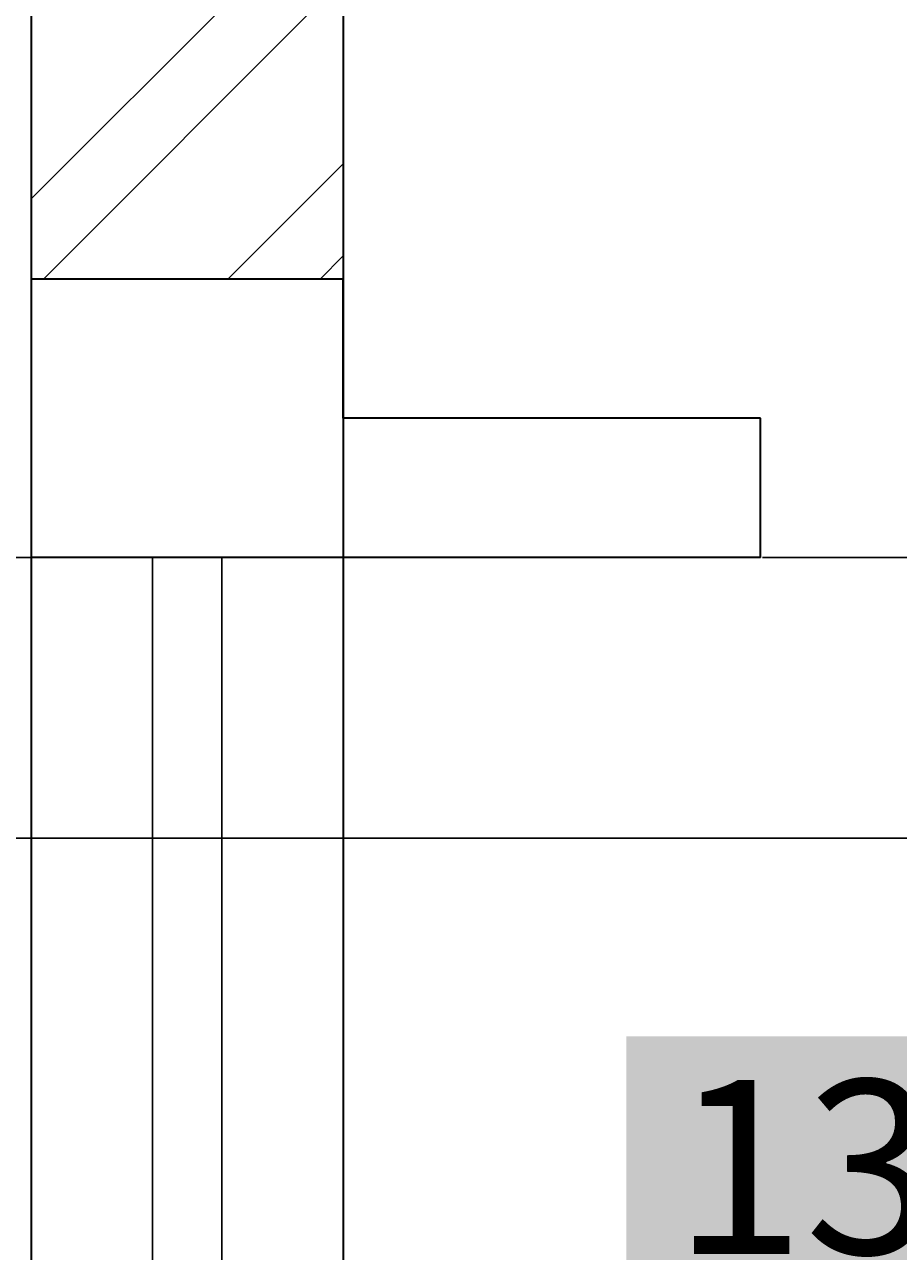
# Model space of a CAD drawing. Units: inches. Extents: x -301 to 715, y -607 to 364.
# Tile 40 of 141: x 134 to 159, y -405 to -370. Entities that reach past the tile are written whole.
import ezdxf

# ---------------------------------------------------------------- set-up
doc = ezdxf.new("R2010")
doc.units = ezdxf.units.IN
doc.header["$MEASUREMENT"] = 0
for name, color, linetype, lineweight in [('A-ANNO-DIMS', 2, 'Continuous', 18), ('A-GLAZ', 2, 'Continuous', 25), ('A-SECT', 1, 'Continuous', 35), ('A-SECT-PATT', 8, 'Continuous', 13)]:
    doc.layers.add(name, color=color, linetype=linetype, lineweight=lineweight)
doc.styles.get("Standard").update_dxf_attribs({"font": 'arial.ttf'})
doc.dimstyles.get("Standard").update_dxf_attribs({"dimtxt": 0.18, "dimasz": 0.18, "dimexe": 0.18, "dimexo": 0.0625, "dimgap": 0.09, "dimtad": 0, "dimtih": 1, "dimtoh": 1, "dimdec": 1, "dimzin": 0, "dimdsep": 46, "dimlunit": 4, "dimtxsty": 'Standard', "dimcen": 0.09, "dimclrd": 3, "dimclre": 4, "dimclrt": 6, "dimadec": 0, "dimazin": 0, "dimtfac": 1, "dimtdec": 1, "dimtofl": 0, "dimtmove": 0, "dimatfit": 3, "dimfxl": 1, "dimtfill": 2, "dimtfillclr": 51, "dimtolj": 1, "dimtzin": 0, "dimarcsym": 0})

# ---------------------------------------------------------------- blocks, each defined once
blk = doc.blocks.new('*D76')
at = {"layer": 'A-ANNO-DIMS', "color": 0, "lineweight": -2, "transparency": 16777216}
for p, q in [((158.28, -324.519), (162.311, -324.519)), ((162.131, -329.519), (162.131, -400.354)), ((162.131, -476.477), (162.131, -405.643)), ((158.28, -481.477), (162.311, -481.477))]:
    blk.add_line(p, q, dxfattribs=at)
at = {"layer": 'A-ANNO-DIMS', "color": 0, "transparency": 16777216}
for points in [[(161.297, -329.519), (162.964, -329.519), (162.131, -324.519)], [(161.297, -476.477), (162.964, -476.477), (162.131, -481.477)]]:
    blk.add_solid(points, dxfattribs=at)
at = {"layer": 'Defpoints', "color": 0, "transparency": 16777216}
for p in [(158.218, -324.519), (162.131, -324.519), (158.218, -481.477)]:
    blk.add_point(p, dxfattribs=at)
at = {"layer": 'A-ANNO-DIMS', "color": 0, "transparency": 16777216, "insert": (162.131, -402.998), "char_height": 5, "attachment_point": 5, "bg_fill": 1, "box_fill_scale": 1.25, "bg_fill_color": 51, "bg_fill_transparency": 0}
blk.add_mtext('\\A1;13\'-1"', dxfattribs=at)
blk = doc.blocks.new('*D81')
at = {"layer": 'A-ANNO-DIMS', "color": 0, "lineweight": -2, "transparency": 16777216}
for p, q in [((155.28, -385.477), (177.024, -385.477)), ((176.844, -390.477), (176.844, -430.835)), ((176.844, -476.477), (176.844, -436.12)), ((158.28, -481.477), (177.024, -481.477))]:
    blk.add_line(p, q, dxfattribs=at)
at = {"layer": 'A-ANNO-DIMS', "color": 0, "transparency": 16777216}
for points in [[(176.011, -390.477), (177.678, -390.477), (176.844, -385.477)], [(176.011, -476.477), (177.678, -476.477), (176.844, -481.477)]]:
    blk.add_solid(points, dxfattribs=at)
at = {"layer": 'Defpoints', "color": 0, "transparency": 16777216}
for p in [(155.218, -385.477), (158.218, -481.477), (176.844, -481.477)]:
    blk.add_point(p, dxfattribs=at)
at = {"layer": 'A-ANNO-DIMS', "color": 0, "transparency": 16777216, "insert": (176.844, -433.477), "char_height": 5, "attachment_point": 5, "bg_fill": 1, "box_fill_scale": 1.25, "bg_fill_color": 51, "bg_fill_transparency": 0}
blk.add_mtext("\\A1;8'", dxfattribs=at)
blk = doc.blocks.new('*D176')
at = {"layer": 'A-ANNO-DIMS', "color": 4, "lineweight": -2, "transparency": 16777216}
for p, q in [((148.28, -324.477), (215.605, -324.477)), ((-15.22, -540.477), (215.605, -540.477))]:
    blk.add_line(p, q, dxfattribs=at)
at = {"layer": 'A-ANNO-DIMS', "color": 3, "lineweight": -2, "transparency": 16777216}
for p, q in [((215.425, -324.657), (215.425, -432.296)), ((215.425, -540.297), (215.425, -432.659))]:
    blk.add_line(p, q, dxfattribs=at)
at = {"layer": 'A-ANNO-DIMS', "color": 3, "transparency": 16777216}
for points in [[(215.395, -324.657), (215.455, -324.657), (215.425, -324.477)], [(215.395, -540.297), (215.455, -540.297), (215.425, -540.477)]]:
    blk.add_solid(points, dxfattribs=at)
at = {"layer": 'Defpoints', "color": 0, "transparency": 16777216}
for p in [(148.218, -324.477), (-15.282, -540.477), (215.425, -540.477)]:
    blk.add_point(p, dxfattribs=at)
at = {"layer": 'A-ANNO-DIMS', "color": 6, "transparency": 16777216, "insert": (215.425, -432.477), "char_height": 0.18, "attachment_point": 5, "bg_fill": 1, "box_fill_scale": 1.25, "bg_fill_color": 51, "bg_fill_transparency": 0}
blk.add_mtext('\\A1;18\'-0"', dxfattribs=at)
blk = doc.blocks.new('*D187')
at = {"layer": 'A-ANNO-DIMS', "color": 4, "lineweight": -2, "transparency": 16777216}
for p, q in [((139.674, -385.477), (-266.112, -385.477)), ((143.155, -439.477), (-266.112, -439.477))]:
    blk.add_line(p, q, dxfattribs=at)
at = {"layer": 'A-ANNO-DIMS', "color": 3, "lineweight": -2, "transparency": 16777216}
for p, q in [((-265.932, -385.657), (-265.932, -412.296)), ((-265.932, -439.297), (-265.932, -412.659))]:
    blk.add_line(p, q, dxfattribs=at)
at = {"layer": 'A-ANNO-DIMS', "color": 3, "transparency": 16777216}
for points in [[(-265.962, -385.657), (-265.902, -385.657), (-265.932, -385.477)], [(-265.962, -439.297), (-265.902, -439.297), (-265.932, -439.477)]]:
    blk.add_solid(points, dxfattribs=at)
at = {"layer": 'Defpoints', "color": 0, "transparency": 16777216}
for p in [(-265.932, -385.477), (139.737, -385.477), (143.218, -439.477)]:
    blk.add_point(p, dxfattribs=at)
at = {"layer": 'A-ANNO-DIMS', "color": 6, "transparency": 16777216, "insert": (-265.932, -412.477), "char_height": 0.18, "attachment_point": 5, "bg_fill": 1, "box_fill_scale": 1.25, "bg_fill_color": 51, "bg_fill_transparency": 0}
blk.add_mtext('\\A1;4\'-6"', dxfattribs=at)
blk = doc.blocks.new('*D200')
at = {"layer": 'A-ANNO-DIMS', "color": 4, "lineweight": -2, "transparency": 16777216}
for p, q in [((412.955, -393.552), (121.926, -393.552)), ((412.955, -489.552), (121.926, -489.552))]:
    blk.add_line(p, q, dxfattribs=at)
at = {"layer": 'A-ANNO-DIMS', "color": 3, "lineweight": -2, "transparency": 16777216}
for p, q in [((122.106, -393.732), (122.106, -441.371)), ((122.106, -489.372), (122.106, -441.734))]:
    blk.add_line(p, q, dxfattribs=at)
at = {"layer": 'A-ANNO-DIMS', "color": 3, "transparency": 16777216}
for points in [[(122.076, -393.732), (122.136, -393.732), (122.106, -393.552)], [(122.076, -489.372), (122.136, -489.372), (122.106, -489.552)]]:
    blk.add_solid(points, dxfattribs=at)
at = {"layer": 'Defpoints', "color": 0, "transparency": 16777216}
for p in [(122.106, -393.552), (413.018, -393.552), (413.018, -489.552)]:
    blk.add_point(p, dxfattribs=at)
at = {"layer": 'A-ANNO-DIMS', "color": 6, "transparency": 16777216, "insert": (122.106, -441.552), "char_height": 0.18, "attachment_point": 5, "bg_fill": 1, "box_fill_scale": 1.25, "bg_fill_color": 51, "bg_fill_transparency": 0}
blk.add_mtext('\\A1;8\'-0"', dxfattribs=at)

msp = doc.modelspace()

# ---------------------------------------------------------------- hatches: boundary and pattern name
at = {"layer": 'A-SECT-PATT'}
h = msp.add_hatch(dxfattribs=at)
h.set_pattern_fill('ANSI32', color=256, scale=15)
h.set_pattern_definition([(45, (10.321, 33.8764), (-3.977476, 3.977476), []), (45, (12.973, 33.8764), (-3.977476, 3.977476), [])])
h.paths.add_polyline_path([(-185.282, -324.477), (-199.282, -324.477), (-199.282, -329.477), (-194.282, -329.477), (-194.282, -353.477), (-185.282, -353.477)])
h.paths.add_polyline_path([(-185.282, -361.477), (-193.904, -361.477), (-193.982, -377.537), (-185.282, -377.537)])
h.paths.add_polyline_path([(143.218, -329.477), (148.218, -329.477), (148.218, -324.477), (134.255, -324.477), (134.255, -353.477), (143.218, -353.477)])
h.paths.add_polyline_path([(143.218, -361.477), (134.255, -361.477), (134.255, -377.477), (143.218, -377.477)])
h.paths.add_polyline_path([(-185.282, -439.477), (-194.282, -439.477), (-194.282, -463.477), (-185.282, -463.477)])
h.paths.add_polyline_path([(-185.282, -471.477), (-194.282, -471.477), (-194.282, -481.477), (-185.282, -481.477)])
h.paths.add_polyline_path([(-185.282, -463.477), (-194.282, -463.477), (-194.282, -466.477), (-185.282, -466.477)])
h.paths.add_polyline_path([(-185.282, -466.477), (-194.282, -466.477), (-194.282, -471.477), (-185.282, -471.477)])
h.paths.add_polyline_path([(-180.282, -481.477), (-185.282, -481.477), (-194.282, -481.477), (-199.282, -481.477), (-199.282, -493.477), (-180.282, -493.477)])
h.paths.add_polyline_path([(-175.282, -493.477), (-180.282, -493.477), (-199.282, -493.477), (-204.282, -493.477), (-204.282, -511.477), (-175.282, -511.477)])
h.paths.add_polyline_path([(-170.282, -511.477), (-175.282, -511.477), (-204.282, -511.477), (-209.282, -511.477), (-209.282, -535.477), (-170.282, -535.477)])
h.paths.add_polyline_path([(-35.282, -463.477), (-41.282, -463.477), (-41.282, -466.477), (-35.282, -466.477)])
h.paths.add_polyline_path([(-35.282, -466.477), (-41.282, -466.477), (-41.282, -471.477), (-35.282, -471.477)])
h.paths.add_polyline_path([(-35.282, -471.477), (-41.282, -471.477), (-41.282, -481.477), (-35.282, -481.477)])
h.paths.add_polyline_path([(-30.282, -481.477), (-46.282, -481.477), (-46.282, -493.477), (-30.282, -493.477)])
h.paths.add_polyline_path([(-25.282, -493.477), (-30.282, -493.477), (-46.282, -493.477), (-51.282, -493.477), (-51.282, -511.477), (-25.282, -511.477)])
h.paths.add_polyline_path([(-20.282, -511.477), (-25.282, -511.477), (-51.282, -511.477), (-56.282, -511.477), (-56.282, -535.477), (-20.282, -535.477)])
h.paths.add_polyline_path([(143.218, -463.477), (134.255, -463.477), (134.255, -466.477), (143.218, -466.477)])
h.paths.add_polyline_path([(143.218, -466.477), (134.255, -466.477), (134.255, -471.477), (143.218, -471.477)])
h.paths.add_polyline_path([(143.218, -471.477), (134.255, -471.477), (134.255, -481.477), (143.218, -481.477)])
h.paths.add_polyline_path([(148.255, -481.477), (143.255, -481.477), (134.255, -481.477), (129.255, -481.477), (129.255, -493.477), (148.255, -493.477)])
h.paths.add_polyline_path([(153.255, -493.477), (148.255, -493.477), (129.255, -493.477), (124.255, -493.477), (124.255, -511.477), (153.255, -511.477)])
h.paths.add_polyline_path([(158.255, -511.477), (153.255, -511.477), (124.255, -511.477), (119.255, -511.477), (119.255, -535.477), (158.255, -535.477)])

# ---------------------------------------------------------------- linework, layer by layer
at = {"layer": 'A-GLAZ'}
for p, q in [((137.737, -439.477), (137.737, -385.477)), ((139.737, -439.477), (139.737, -385.477))]:
    msp.add_line(p, q, dxfattribs=at)
at = {"layer": 'A-SECT'}
for p, q in [((143.218, -353.477), (143.218, -481.477)), ((134.255, -361.477), (134.255, -481.477)), ((143.218, -377.477), (134.255, -377.477)), ((143.218, -381.477), (143.218, -377.477)), ((155.218, -381.477), (143.218, -381.477)), ((155.218, -385.477), (155.218, -381.477)), ((155.218, -385.477), (134.255, -385.477))]:
    msp.add_line(p, q, dxfattribs=at)

# ---------------------------------------------------------------- dimensions: what is measured, and where the dimension line sits
at = {"layer": 'A-ANNO-DIMS'}
for base, p1, p2, override, picture, middle in [((215.425, -540.477), (148.218, -324.477), (-15.282, -540.477), {"dimdec": 1, "dimlfac": 1, "dimrnd": 0, "dimzin": 1, "dimdsep": 46, "dimlunit": 4, "dimfrac": 2}, '*D176', (215.425, -432.477)), ((162.131, -324.519), (158.218, -481.477), (158.218, -324.519), {"dimtxt": 5, "dimasz": 5, "dimclrd": 0, "dimclre": 0, "dimclrt": 0}, '*D76', (162.131, -402.998)), ((-265.932, -385.477), (143.218, -439.477), (139.737, -385.477), {"dimdec": 1, "dimlfac": 1, "dimrnd": 0, "dimzin": 1, "dimdsep": 46, "dimlunit": 4, "dimfrac": 2}, '*D187', (-265.932, -412.477)), ((176.844, -481.477), (155.218, -385.477), (158.218, -481.477), {"dimtxt": 5, "dimasz": 5, "dimclrd": 0, "dimclre": 0, "dimclrt": 0}, '*D81', (176.844, -433.477)), ((122.106, -393.552), (413.018, -489.552), (413.018, -393.552), {"dimdec": 1, "dimlfac": 1, "dimrnd": 0, "dimzin": 1, "dimdsep": 46, "dimlunit": 4, "dimfrac": 2}, '*D200', (122.106, -441.552))]:
    dim = msp.add_linear_dim(base=base, p1=p1, p2=p2, angle=90, dimstyle='Standard', override=override, dxfattribs=at)
    dim.commit()
    dim.dimension.update_dxf_attribs({"geometry": picture, "text_midpoint": middle})

doc.saveas('drawing.dxf')
